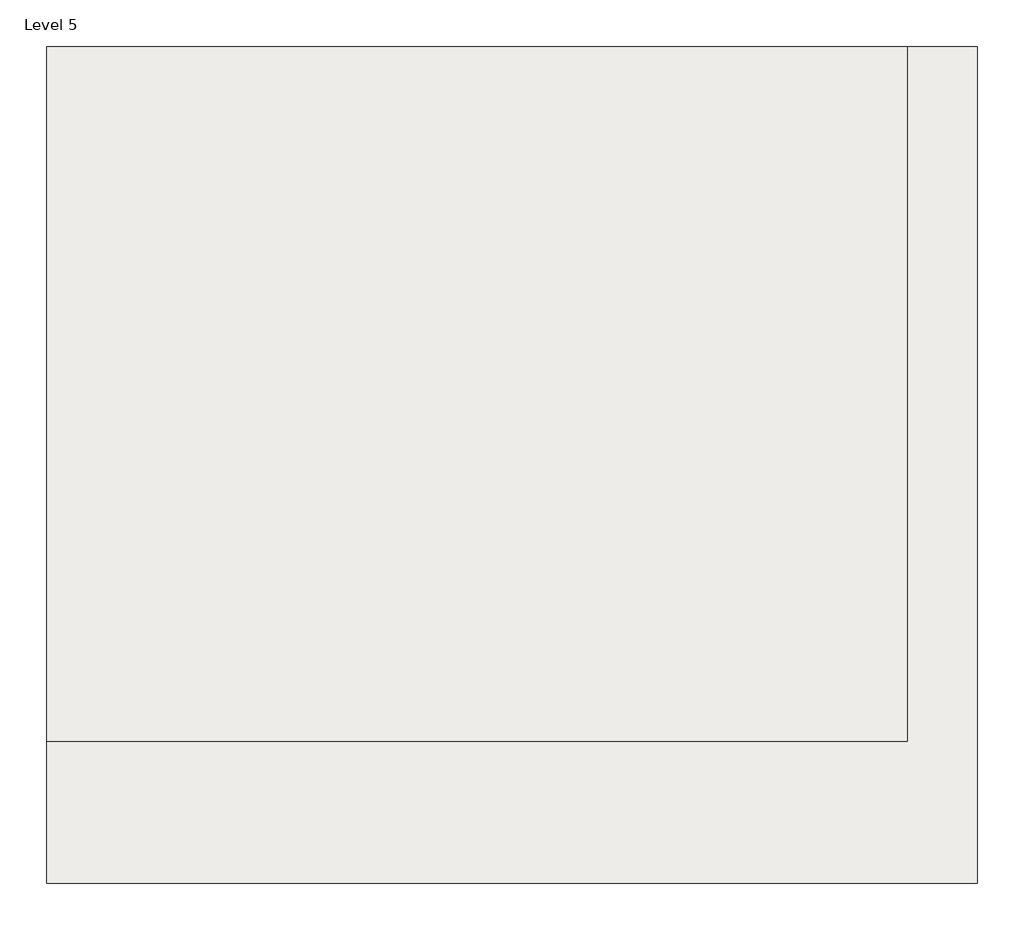
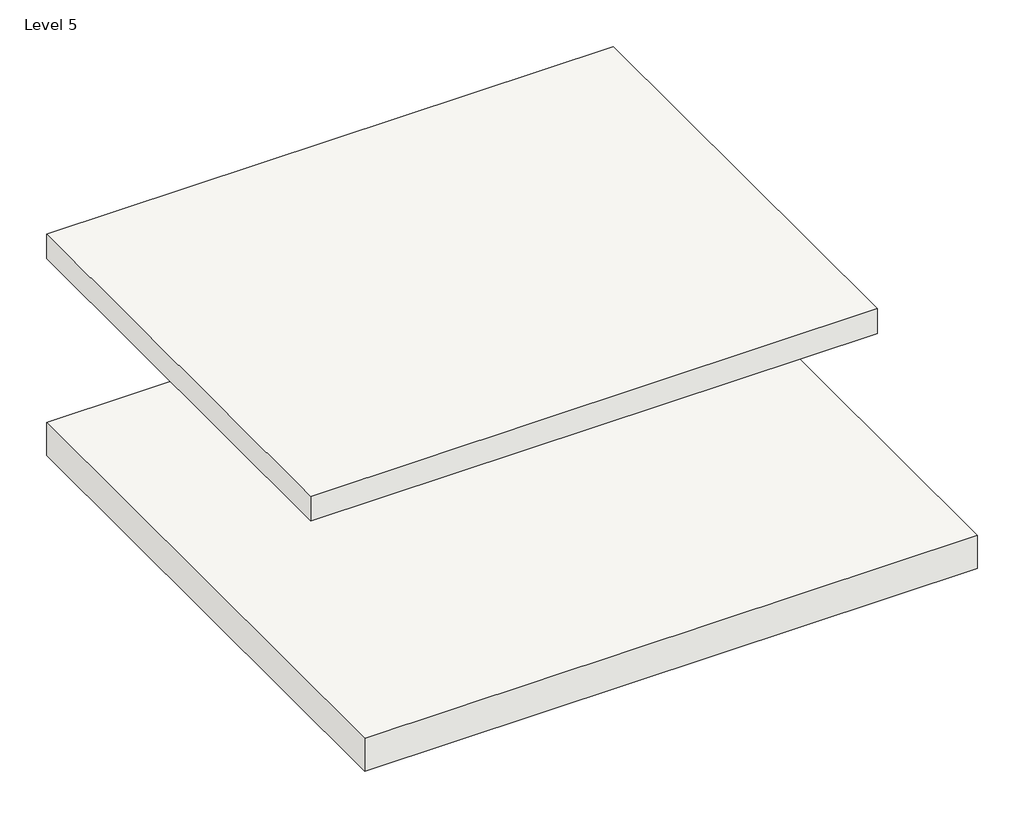
# One storey: 2 roofs.
"""IFC4 building model written with IfcOpenShell, lengths in millimetres."""

from ifc_helpers import new_model, si_unit, frame, origin, place, context, project, spatial, polyline, outline, extrude, element, save

model = new_model("IFC4")

# Units and contexts
model_context = context("Model", 3, world=origin())
ifc_project = project(units=[si_unit("LENGTHUNIT", "METRE", prefix="MILLI")], contexts=[model_context])

# Site, building, storey
site = spatial("IfcSite", under=ifc_project)
building = spatial("IfcBuilding", under=site)
storey = spatial("IfcBuildingStorey", under=building, Name="Level 5", Elevation=14630.4)

# Roofs
placement = place(None, origin())
element("IfcRoof", 1, ObjectType="Generic - 12\"", at=placement, inside=storey, context=model_context, shape_type="SweptSolid", body=[
    extrude(outline(polyline([(-8705.5936733, 8294.4419215), (-3320.7936733, 8294.4419215), (-3320.7936733, 3455.7419215), (-8705.5936733, 3455.7419215), (-8705.5936733, 8294.4419215)])), frame((0.0, 0.0, 12801.6), z_axis=(0.0, 0.0, 1.0), x_axis=(1.0, 0.0, 0.0)), (0.0, 0.0, 1.0), 304.8),
])
element("IfcRoof", 2, ObjectType="Generic - 9\"", at=placement, inside=storey, context=model_context, shape_type="SweptSolid", body=[
    extrude(outline(polyline([(-8705.5936733, 4274.8919215), (-8705.5936733, 8294.4419215), (-3727.1936733, 8294.4419215), (-3727.1936733, 4274.8919215), (-8705.5936733, 4274.8919215)])), frame((0.0, 0.0, 14630.4), z_axis=(0.0, 0.0, 1.0), x_axis=(1.0, 0.0, 0.0)), (0.0, 0.0, 1.0), 228.6),
])

save(model, "model.ifc")

# Revit data of these elements
# Type "Generic - 12\""
#   Assembly Code = "B1020"
#   Layers, outside or top first: 1' - 0" no material (function 1)
# Type "Generic - 9\""
#   Assembly Code = "B1020"
#   Layers, outside or top first: 0' - 9" no material (function 1)
# Element 1 (IfcRoof, "Generic - 12\"")
#   built-in parameter 1001705 = 43 (stored number, unit not read)
#   built-in parameter 1001701 = -6 (stored number, unit not read)
#   built-in parameter 1001710 = 33615
#   Phase Created = New Construction
#   Materials on its faces: "Default Roof"
# Element 2 (IfcRoof, "Generic - 9\"")
#   built-in parameter 1001705 = 48.75 (stored number, unit not read)
#   built-in parameter 1001710 = 33615
#   Phase Created = New Construction
#   Materials on its faces: "Default Roof"
# Materials
#   "Default Roof": colour RGB 88 101 114, transparency 0
